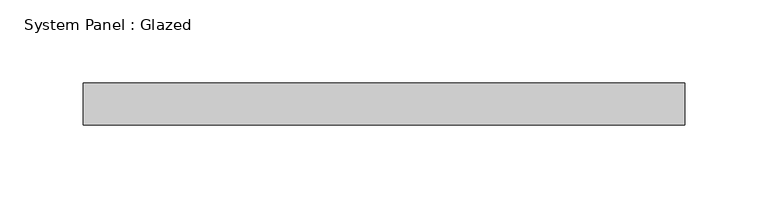
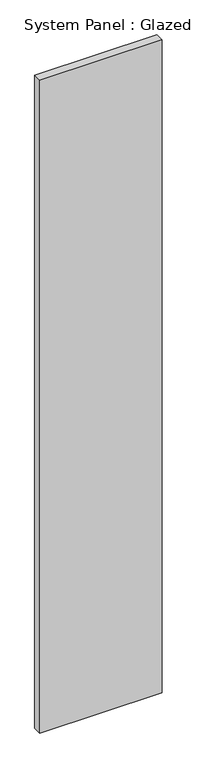
"""IFC4 building model written with IfcOpenShell, lengths in millimetres: plate geometry, System Panel : Glazed."""

from ifc_helpers import new_model, si_unit, origin, origin_with_axes, place, context, project, spatial, polyline, outline, extrude, source, transform, mapped, element, save


def system_panel_glazed_a2bc0953(model_context):
    return source(origin(), model_context, "Body", "SweptSolid", [
        extrude(outline(polyline([(180.975, 19.05), (-180.975, 19.05), (-180.975, 44.45), (180.975, 44.45), (180.975, 19.05)])), origin_with_axes(), (0.0, 0.0, 1.0), 2038.35),
    ])


if __name__ == "__main__":
    model = new_model("IFC4")
    model_context = context("Model", 3, world=origin())
    ifc_project = project(units=[si_unit("LENGTHUNIT", "METRE", prefix="MILLI")], contexts=[model_context])
    site = spatial("IfcSite", under=ifc_project)
    building = spatial("IfcBuilding", under=site)
    placement = place(None, origin())
    system_panel_glazed_shape = system_panel_glazed_a2bc0953(model_context)
    element("IfcPlate", 1, ObjectType="System Panel : Glazed", at=placement, inside=building, context=model_context, shape_type="MappedRepresentation", body=[
        mapped(system_panel_glazed_shape, transform((0.0, 0.0, 0.0), x_axis=(1.0, 0.0, 0.0), y_axis=(0.0, 1.0, 0.0), z_axis=(0.0, 0.0, 1.0))),
    ])
    save(model, "model.ifc")

# Revit data of these elements
# Type "System Panel : Glazed"
#   Construction Type Id = "GSP4R"
#   Analytic Construction = "1/8 in Pilkington single glazing"
#   Visual Light Transmittance = 0.9
#   Solar Heat Gain Coefficient = 0.86
#   Heat Transfer Coefficient (U) = 1.18115 BTU/(h·ft²·°F)
#   Define Thermal Properties by = 1
# Element 1 (IfcPlate, "System Panel : Glazed")
#   Materials on its faces: "Glass"
# Materials
#   "Glass": class "Glass", colour RGB 0 128 192, transparency 0.75, Description = "Soda Lime Glass", Cost = 0
